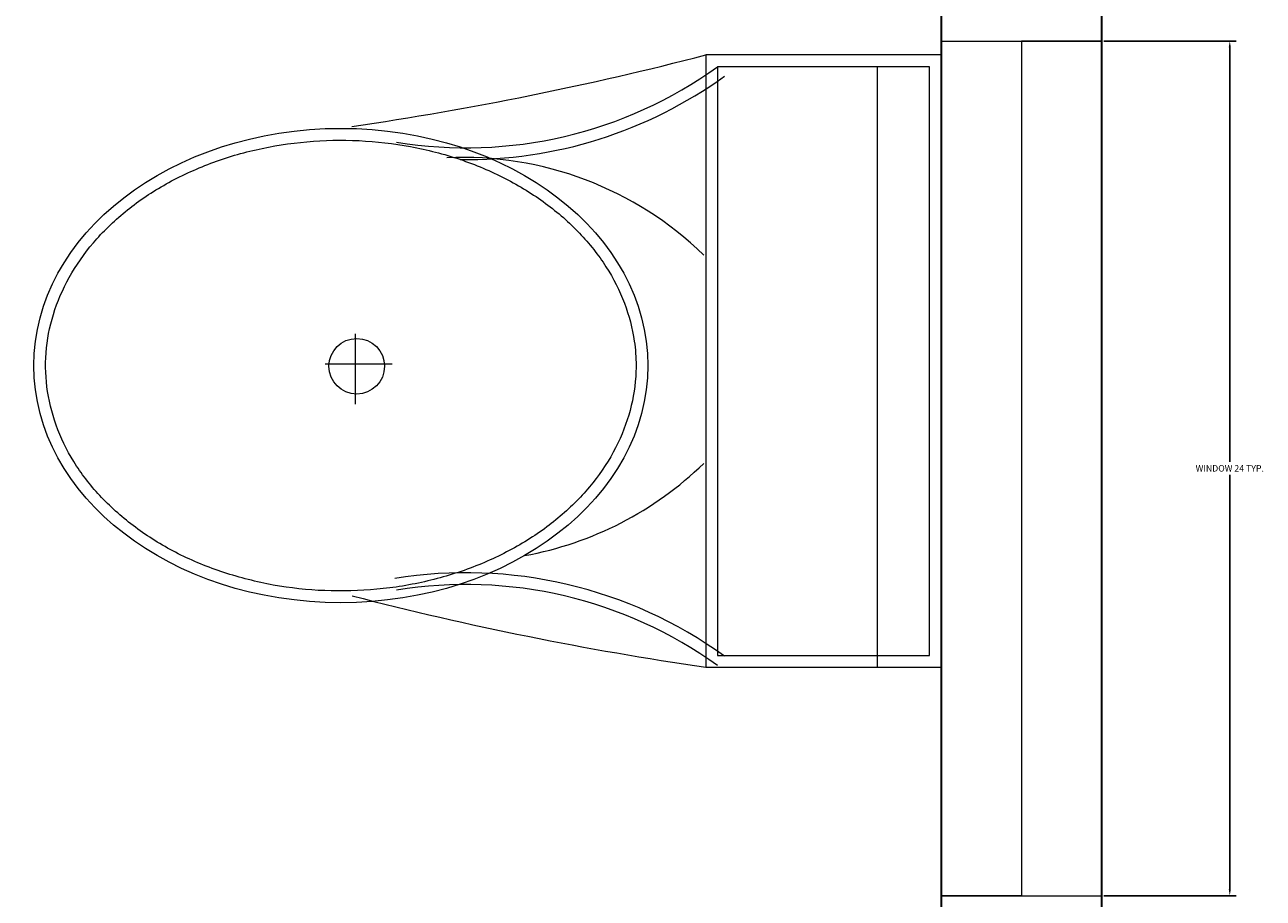
# Model space of a CAD drawing. Units: inches. Extents: x 1088 to 1703, y 668 to 1875.
# Tile 37 of 45: x 1560 to 1595, y 1629 to 1654. Entities that reach past the tile are written whole.
import ezdxf

# ---------------------------------------------------------------- set-up
doc = ezdxf.new("R2010")
doc.units = ezdxf.units.IN
for name, color, linetype, lineweight in [('A-ANNO-DIMS', 2, 'Continuous', 18), ('A-FLOR-FIXT', 8, 'Continuous', 18), ('A-GLAZ', 4, 'Continuous', 18), ('A-WALL', 7, 'Continuous', 35)]:
    doc.layers.add(name, color=color, linetype=linetype, lineweight=lineweight)
doc.styles.get("Standard").update_dxf_attribs({"font": 'arial.ttf'})
doc.dimstyles.get("Standard").update_dxf_attribs({"dimtxt": 0.18, "dimasz": 0.18, "dimexe": 0.18, "dimexo": 0.0625, "dimgap": 0.09, "dimtad": 0, "dimtih": 1, "dimtoh": 1, "dimdec": 4, "dimzin": 0, "dimdsep": 46, "dimtxsty": 'Standard', "dimcen": 0.09, "dimadec": 0, "dimazin": 0, "dimtfac": 1, "dimtdec": 4, "dimtofl": 0, "dimtmove": 0, "dimatfit": 3, "dimfxl": 1, "dimtolj": 1, "dimtzin": 0, "dimarcsym": 0})

# ---------------------------------------------------------------- blocks, each defined once
blk = doc.blocks.new('A$C31115884')
for p, q in [((257.5, 466.4), (257.5, 523.2)), ((283.1, 497.7), (223.4, 497.7)), ((0, 200), (0, 0)), ((520, 200), (0, 200)), ((520, 0), (520, 200)), ((10, 190), (10, 10)), ((510, 190), (10, 190)), ((510, 10), (510, 190)), ((510, 54.5), (0, 54.5)), ((10, 10), (510, 10)), ((0, 0), (520, 0))]:
    blk.add_line(p, q)
blk.add_circle((255.6, 496.4), 23.6)
for centre, radius, start, end in [((2777.7, -204.6), 2807, 165.4549, 171.7133), ((3237, 905), 2807, 188.2867, 194.5451), ((-294.5, 403.3), 374.7, 324.2091, 9.3499), ((-294.5, 403.3), 364.7, 324.2091, 9.3499), ((805.8, 403.3), 364.7, 170.6501, 215.7909), ((139.5, 406.2), 293.5, 315.8436, 2.6563), ((805.8, 403.3), 374.7, 179.2036, 215.7909), ((383.6, 406.2), 293.5, 190.2774, 224.1564)]:
    blk.add_arc(centre, radius, start, end)
blk.add_ellipse((256.2, 509.9), major_axis=(0, -260.7), ratio=0.772727)
blk.add_open_spline([(256.2, 259.2), (263.1, 259.2), (270, 259.7), (287.8, 262.3), (298.7, 265.1), (319.9, 273.1), (330.2, 278.4), (350.1, 291.1), (359.7, 298.7), (377.7, 315.9), (386.2, 325.5), (401.7, 346.6), (408.8, 358.1), (421.3, 382.5), (426.8, 395.5), (435.9, 422.4), (439.5, 436.4), (444.8, 465.1), (446.5, 479.7), (447.9, 509.2), (447.6, 524), (445, 553.3), (442.7, 567.8), (436.3, 596), (432.1, 609.7), (421.9, 636), (416, 648.6), (402.5, 672.1), (395, 683), (378.6, 703), (369.8, 712.1), (351.1, 728), (341.3, 734.8), (320.9, 746.2), (310.4, 750.7), (288.9, 757.3), (278, 759.4), (256, 761), (245, 760.6), (223.1, 757.2), (212.3, 754.3), (191.1, 746.1), (180.8, 740.7), (160.9, 727.8), (151.4, 720.1), (133.5, 702.7), (125.1, 693), (109.6, 671.7), (102.6, 660.2), (90.2, 635.7), (84.9, 622.7), (76, 595.6), (72.4, 581.6), (67.2, 552.9), (65.6, 538.2), (64.4, 508.8), (64.8, 494), (67.5, 464.7), (69.9, 450.2), (76.6, 422), (80.8, 408.3), (91.1, 382.2), (97.2, 369.7), (110.8, 346.3), (118.4, 335.4), (134.8, 315.6), (143.7, 306.7), (162.4, 290.9), (172.3, 284.2), (192.8, 273), (203.3, 268.6), (224.8, 262.2), (235.8, 260.2), (249.9, 259.3), (253, 259.2), (256.2, 259.2)], degree=3, knots=[0, 0, 0, 0, 0.110105, 0.110105, 0.285049, 0.285049, 0.459994, 0.459994, 0.634938, 0.634938, 0.809882, 0.809882, 0.984827, 0.984827, 1.159771, 1.159771, 1.334715, 1.334715, 1.50966, 1.50966, 1.684604, 1.684604, 1.859549, 1.859549, 2.034493, 2.034493, 2.209437, 2.209437, 2.384382, 2.384382, 2.559326, 2.559326, 2.73427, 2.73427, 2.909215, 2.909215, 3.084159, 3.084159, 3.259103, 3.259103, 3.434048, 3.434048, 3.608992, 3.608992, 3.783936, 3.783936, 3.958881, 3.958881, 4.133825, 4.133825, 4.30877, 4.30877, 4.483714, 4.483714, 4.658658, 4.658658, 4.833603, 4.833603, 5.008547, 5.008547, 5.183491, 5.183491, 5.358436, 5.358436, 5.53338, 5.53338, 5.708324, 5.708324, 5.883269, 5.883269, 6.058213, 6.058213, 6.233158, 6.233158, 6.283185, 6.283185, 6.283185, 6.283185])
blk = doc.blocks.new('WIN-24-OPPOSED-RETURN')
for p, q in [((0, 24), (4.5, 24)), ((4.5, 24), (2.25, 24)), ((2.25, 24), (2.25, 0)), ((2.25, 0), (0, 0)), ((0, 0), (4.5, 0))]:
    blk.add_line(p, q)
blk = doc.blocks.new('*D20')
at = {"layer": 'A-ANNO-DIMS', "color": 0, "lineweight": -2, "transparency": 16777216}
for p, q in [((1590.407, 1653.317), (1594.125, 1653.317)), ((1593.945, 1653.137), (1593.945, 1641.5)), ((1593.945, 1629.497), (1593.945, 1641.134)), ((1590.407, 1629.317), (1594.125, 1629.317))]:
    blk.add_line(p, q, dxfattribs=at)
at = {"layer": 'A-ANNO-DIMS', "color": 0, "transparency": 16777216}
for points in [[(1593.915, 1653.137), (1593.975, 1653.137), (1593.945, 1653.317)], [(1593.915, 1629.497), (1593.975, 1629.497), (1593.945, 1629.317)]]:
    blk.add_solid(points, dxfattribs=at)
at = {"layer": 'Defpoints', "color": 0, "transparency": 16777216}
for p in [(1590.345, 1653.317), (1593.945, 1653.317), (1590.345, 1629.317)]:
    blk.add_point(p, dxfattribs=at)
at = {"layer": 'A-ANNO-DIMS', "color": 0, "transparency": 16777216, "insert": (1593.945, 1641.317), "char_height": 0.18, "attachment_point": 5}
blk.add_mtext('\\A1;WINDOW 24 TYP.', dxfattribs=at)
blk = doc.blocks.new('*D21')
at = {"layer": 'A-ANNO-DIMS', "color": 0, "lineweight": -2, "transparency": 16777216}
for p, q in [((1585.845, 1629.254), (1585.845, 1625.537)), ((1590.345, 1629.254), (1590.345, 1625.537)), ((1586.025, 1625.717), (1587.637, 1625.717)), ((1590.165, 1625.717), (1588.553, 1625.717))]:
    blk.add_line(p, q, dxfattribs=at)
at = {"layer": 'A-ANNO-DIMS', "color": 0, "transparency": 16777216}
for points in [[(1586.025, 1625.747), (1586.025, 1625.687), (1585.845, 1625.717)], [(1590.165, 1625.747), (1590.165, 1625.687), (1590.345, 1625.717)]]:
    blk.add_solid(points, dxfattribs=at)
at = {"layer": 'Defpoints', "color": 0, "transparency": 16777216}
for p in [(1585.845, 1629.317), (1590.345, 1629.317), (1590.345, 1625.717)]:
    blk.add_point(p, dxfattribs=at)
at = {"layer": 'A-ANNO-DIMS', "color": 0, "transparency": 16777216, "insert": (1588.095, 1625.717), "char_height": 0.18, "attachment_point": 5}
blk.add_mtext('\\A1;5 TYP.', dxfattribs=at)
blk = doc.blocks.new('*D32')
at = {"layer": 'A-ANNO-DIMS', "color": 0, "lineweight": -2, "transparency": 16777216}
for p, q in [((1550.595, 1373.121), (1550.595, 1857.788)), ((1550.775, 1857.608), (1567.825, 1857.608)), ((1585.665, 1857.608), (1568.614, 1857.608)), ((1585.845, 1360.983), (1585.845, 1857.788))]:
    blk.add_line(p, q, dxfattribs=at)
at = {"layer": 'A-ANNO-DIMS', "color": 0, "transparency": 16777216}
for points in [[(1550.775, 1857.638), (1550.775, 1857.578), (1550.595, 1857.608)], [(1585.665, 1857.638), (1585.665, 1857.578), (1585.845, 1857.608)]]:
    blk.add_solid(points, dxfattribs=at)
at = {"layer": 'Defpoints', "color": 0, "transparency": 16777216}
for p in [(1585.845, 1857.608), (1550.595, 1373.058), (1585.845, 1360.921)]:
    blk.add_point(p, dxfattribs=at)
at = {"layer": 'A-ANNO-DIMS', "color": 0, "transparency": 16777216, "insert": (1568.22, 1857.608), "char_height": 0.18, "attachment_point": 5}
blk.add_mtext('\\A1;35.25', dxfattribs=at)

msp = doc.modelspace()

# ---------------------------------------------------------------- linework, layer by layer
at = {"layer": 'A-WALL'}
for p, q in [((1590.345, 1673.058), (1590.345, 1539.558)), ((1585.845, 1668.558), (1585.845, 1544.058)), ((1585.845, 1668.558), (1585.845, 1608.558))]:
    msp.add_line(p, q, dxfattribs=at)

# ---------------------------------------------------------------- block references
at = {"layer": 'A-FLOR-FIXT', "xscale": 0.0330640103915726, "yscale": 0.0330640103915726, "zscale": 0.0330640103915726, "rotation": 89.99999999999996}
msp.add_blockref('A$C31115884', (1585.845, 1635.733), dxfattribs=at)
at = {"layer": 'A-GLAZ'}
msp.add_blockref('WIN-24-OPPOSED-RETURN', (1585.845, 1629.317), dxfattribs=at)

# ---------------------------------------------------------------- dimensions: what is measured, and where the dimension line sits
at = {"layer": 'A-ANNO-DIMS'}
dim = msp.add_linear_dim(base=(1585.845, 1857.608), p1=(1550.595, 1373.058), p2=(1585.845, 1360.921), dimstyle='Standard', override={"dimdec": 2, "dimlfac": 1, "dimrnd": 0, "dimzin": 0, "dimdsep": 46, "dimlunit": 2}, dxfattribs=at)
dim.commit()
dim.dimension.update_dxf_attribs({"geometry": '*D32', "text_midpoint": (1568.22, 1857.608)})
dim = msp.add_linear_dim(base=(1593.945, 1653.317), p1=(1590.345, 1629.317), p2=(1590.345, 1653.317), angle=90, text='WINDOW <> TYP.', dimstyle='Standard', override={"dimdec": 0, "dimlfac": 1, "dimrnd": 0, "dimzin": 0, "dimdsep": 46, "dimlunit": 2}, dxfattribs=at)
dim.commit()
dim.dimension.update_dxf_attribs({"geometry": '*D20', "text_midpoint": (1593.945, 1641.317)})
dim = msp.add_linear_dim(base=(1590.344800082, 1625.716851167), p1=(1585.844800082, 1629.316851167), p2=(1590.344800082, 1629.316851167), text='<> TYP.', dimstyle='Standard', override={"dimdec": 0, "dimlfac": 1, "dimrnd": 0, "dimzin": 0, "dimdsep": 46, "dimlunit": 2}, dxfattribs=at)
dim.commit()
dim.dimension.update_dxf_attribs({"geometry": '*D21', "text_midpoint": (1588.094800082, 1625.716851167)})

doc.saveas('drawing.dxf')
